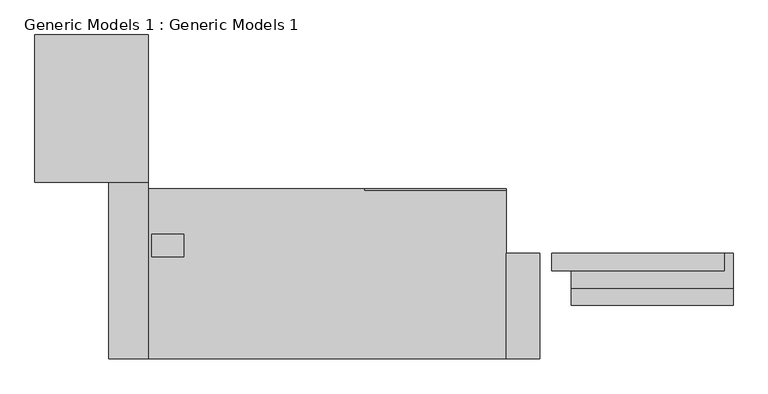
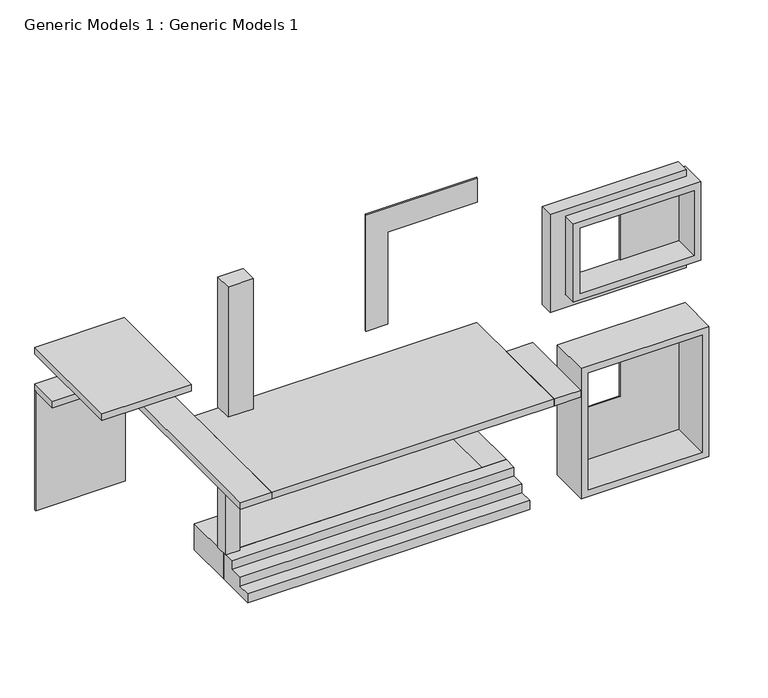
"""IFC4 building model written with IfcOpenShell, lengths in millimetres: proxy geometry, Generic Models 1 : Generic Models 1."""

from ifc_helpers import new_model, si_unit, frame, origin, origin_with_axes, place, context, project, spatial, polyline, outline, extrude, source, transform, mapped, element, save


def generic_models_1_generic_models_1_206d5355(model_context):
    return source(origin(), model_context, "Body", "SweptSolid", [
        extrude(outline(polyline([(5359.4, -3596.6915113), (5359.4, -1615.4915113), (5929.6731526, -1615.4915113), (5929.6731526, -4086.3703016), (3200.4, -4086.3703016), (3200.4, -3596.6915113), (5359.4, -3596.6915113)])), frame((0.0, 1462.8599631, 0.0), z_axis=(0.0, 1.0, 0.0), x_axis=(0.0, 0.0, 1.0)), (0.0, 0.0, 1.0), 25.4),
        extrude(outline(polyline([(609.6, 892.7584887), (609.6, -326.4415113), (-609.6, -326.4415113), (-609.6, 2194.5084887), (609.6, 2194.5084887), (2133.6, 2194.5084887), (2133.6, 892.7584887), (609.6, 892.7584887)])), frame((0.0, 338.9099631, 0.0), z_axis=(0.0, 1.0, 0.0), x_axis=(0.0, 0.0, 1.0)), (0.0, 0.0, 1.0), 25.4),
        extrude(outline(polyline([(-7863.8915113, 4148.9099631), (-9845.0915113, 4148.9099631), (-9845.0915113, 4174.3099631), (-7863.8915113, 4174.3099631), (-7863.8915113, 4148.9099631)])), frame((0.0, 0.0, -609.6), z_axis=(0.0, 0.0, 1.0), x_axis=(1.0, 0.0, 0.0)), (0.0, 0.0, 1.0), 2800.9131177),
        extrude(outline(polyline([(-7247.9415113, 692.1711906), (-7247.9415113, 298.4711906), (-7806.7415113, 298.4711906), (-7806.7415113, 692.1711906), (-7247.9415113, 692.1711906)])), frame((0.0, 0.0, 3200.4), z_axis=(0.0, 0.0, 1.0), x_axis=(1.0, 0.0, 0.0)), (0.0, 0.0, 1.0), 3048.0),
        extrude(outline(polyline([(-7863.8915113, 1602.5599631), (-9845.0915113, 1602.5599631), (-9845.0915113, 4174.3099631), (-7863.8915113, 4174.3099631), (-7863.8915113, 1602.5599631)])), frame((0.0, 0.0, 3048.0), z_axis=(0.0, 0.0, 1.0), x_axis=(1.0, 0.0, 0.0)), (0.0, 0.0, 1.0), 152.4),
        extrude(outline(polyline([(5486.4, -478.8415113), (5486.4, 2194.5084887), (5638.8, 2194.5084887), (5638.8, -815.3915113), (3352.8, -815.3915113), (3352.8, 2194.5084887), (3657.6, 2194.5084887), (3657.6, -478.8415113), (5486.4, -478.8415113)])), frame((0.0, 59.5099631, 0.0), z_axis=(0.0, 1.0, 0.0), x_axis=(0.0, 0.0, 1.0)), (0.0, 0.0, 1.0), 304.8),
        extrude(outline(polyline([(2194.5084887, 338.9099631), (892.7584887, 338.9099631), (892.7584887, 364.3099631), (2194.5084887, 364.3099631), (2194.5084887, 338.9099631)])), frame((0.0, 0.0, 3810.0), z_axis=(0.0, 0.0, 1.0), x_axis=(1.0, 0.0, 0.0)), (0.0, 0.0, 1.0), 1524.0),
        extrude(outline(polyline([(5486.4, 2346.9084887), (5486.4, -478.8415113), (3657.6, -478.8415113), (3657.6, 2346.9084887), (5486.4, 2346.9084887)]), holes=[polyline([(5334.0, 2194.5084887), (3810.0, 2194.5084887), (3810.0, -326.4415113), (5334.0, -326.4415113), (5334.0, 2194.5084887)])]), frame((0.0, -245.2900369, 0.0), z_axis=(0.0, 1.0, 0.0), x_axis=(0.0, 0.0, 1.0)), (0.0, 0.0, 1.0), 609.6),
        extrude(outline(polyline([(2286.0, 2346.9084887), (2286.0, -478.8415113), (-762.0, -478.8415113), (-762.0, 2346.9084887), (2286.0, 2346.9084887)]), holes=[polyline([(2133.6, 2194.5084887), (-609.6, 2194.5084887), (-609.6, -326.4415113), (2133.6, -326.4415113), (2133.6, 2194.5084887)])]), frame((0.0, -549.3228083, 0.0), z_axis=(0.0, 1.0, 0.0), x_axis=(0.0, 0.0, 1.0)), (0.0, 0.0, 1.0), 913.6327714),
        extrude(outline(polyline([(-7863.8915113, 3504.5599355), (-9845.0915113, 3504.5599355), (-9845.0915113, 4174.3099631), (-7863.8915113, 4174.3099631), (-7863.8915113, 3504.5599355)])), frame((0.0, 0.0, 2191.3131177), z_axis=(0.0, 0.0, 1.0), x_axis=(1.0, 0.0, 0.0)), (0.0, 0.0, 1.0), 152.4),
        extrude(outline(polyline([(-7559.0915113, 284.5973944), (-7863.8915113, 284.5973944), (-7863.8915113, 589.3973944), (-7559.0915113, 589.3973944), (-7559.0915113, 284.5973944)])), origin_with_axes(), (0.0, 0.0, 1.0), 2378.1713747),
        extrude(outline(polyline([(365.0771917, -609.6), (-549.3228083, -609.6), (-549.3228083, -406.4), (-244.5228083, -406.4), (-244.5228083, -203.2), (60.2771917, -203.2), (60.2771917, 0.0), (365.0771917, 0.0), (365.0771917, -609.6)])), frame((-7863.8915113, 0.0, 0.0), z_axis=(1.0, 0.0, 0.0), x_axis=(0.0, 1.0, 0.0)), (0.0, 0.0, 1.0), 6248.4),
        extrude(outline(polyline([(0.0, -1615.4915113), (0.0, -2142.5415113), (0.0, -7863.8915113), (-609.6, -7863.8915113), (-609.6, -1615.4915113), (0.0, -1615.4915113)])), frame((0.0, 364.3099631, 0.0), z_axis=(0.0, 1.0, 0.0), x_axis=(0.0, 0.0, 1.0)), (0.0, 0.0, 1.0), 1123.95),
        extrude(outline(polyline([(-1026.5217933, 364.3099631), (-1026.5217933, -1477.1683541), (-1615.4915113, -1477.1683541), (-1615.4915113, 364.3099631), (-1026.5217933, 364.3099631)])), frame((0.0, 0.0, 2378.1713747), z_axis=(0.0, 0.0, 1.0), x_axis=(1.0, 0.0, 0.0)), (0.0, 0.0, 1.0), 152.4),
        extrude(outline(polyline([(-8558.9751487, -1477.1683541), (-8558.9751487, 4174.3099631), (-7863.8915113, 4174.3099631), (-7863.8915113, -1477.1683541), (-8558.9751487, -1477.1683541)])), frame((0.0, 0.0, 2378.1713747), z_axis=(0.0, 0.0, 1.0), x_axis=(1.0, 0.0, 0.0)), (0.0, 0.0, 1.0), 152.4),
        extrude(outline(polyline([(-1615.4915113, -1477.1683541), (-7863.8915113, -1477.1683541), (-7863.8915113, 1488.2599631), (-1615.4915113, 1488.2599631), (-1615.4915113, -1477.1683541)])), frame((0.0, 0.0, 2378.1713747), z_axis=(0.0, 0.0, 1.0), x_axis=(1.0, 0.0, 0.0)), (0.0, 0.0, 1.0), 152.4),
    ])


if __name__ == "__main__":
    model = new_model("IFC4")
    model_context = context("Model", 3, world=origin())
    ifc_project = project(units=[si_unit("LENGTHUNIT", "METRE", prefix="MILLI")], contexts=[model_context])
    site = spatial("IfcSite", under=ifc_project)
    building = spatial("IfcBuilding", under=site)
    placement = place(None, origin())
    generic_models_1_generic_models_1_shape = generic_models_1_generic_models_1_206d5355(model_context)
    element("IfcBuildingElementProxy", 1, Name="Generic Models 1 : Generic Models 1", ObjectType="Generic Models 1 : Generic Models 1", at=placement, inside=building, context=model_context, shape_type="MappedRepresentation", body=[
        mapped(generic_models_1_generic_models_1_shape, transform((0.0, 0.0, 0.0), x_axis=(1.0, 0.0, 0.0), y_axis=(0.0, 1.0, 0.0), z_axis=(0.0, 0.0, 1.0))),
    ])
    save(model, "model.ifc")

# Revit data of these elements
# Element 1 (IfcBuildingElementProxy, "Generic Models 1 : Generic Models 1")
#   Materials on its faces: "Laminate, Ivory, Matte", "Wood Planks"
# Materials
#   "Laminate, Ivory, Matte": class "Plastic", colour RGB 247 247 239, transparency 0, Description = "Plastic Laminate - Ivory, Matte", Cost = 0
#   "Wood Planks": class "Wood", colour RGB 193 160 115, transparency 0, Description = "Physical material.", Cost = 0
